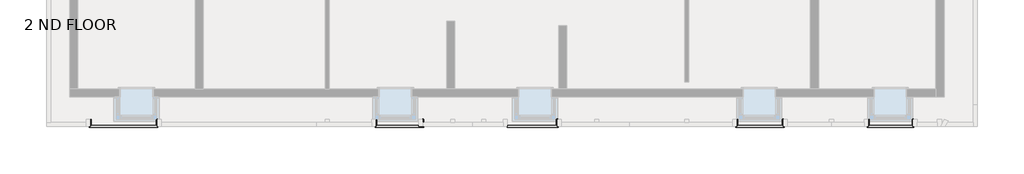
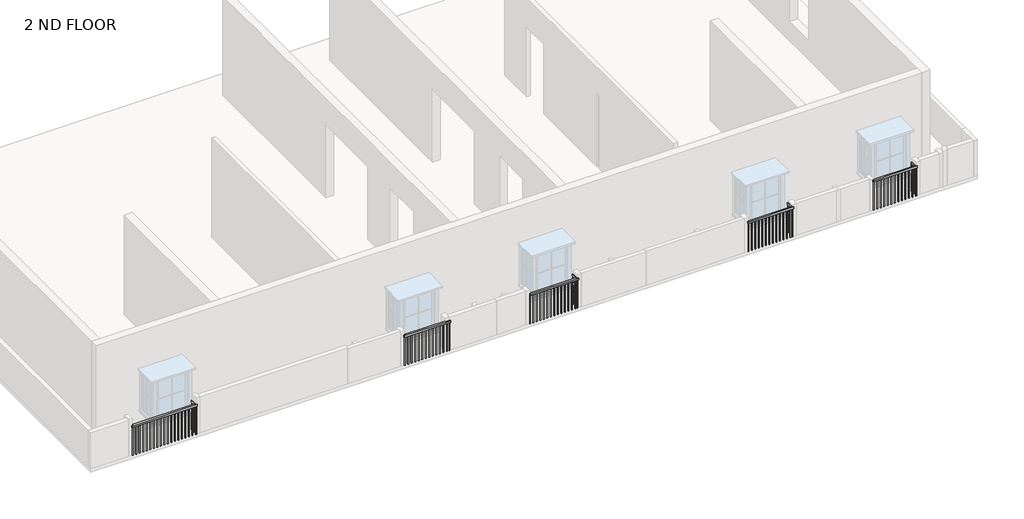
# One storey, part 3 of 7: 5 railings.
"""IFC4 building model written with IfcOpenShell, lengths in millimetres."""

from ifc_helpers import new_model, si_unit, frame, origin, place, context, project, spatial, polyline, outline, extrude, faceted_brep, element, save

model = new_model("IFC4")

# Units and contexts
model_context = context("Model", 3, world=origin())
ifc_project = project(units=[si_unit("LENGTHUNIT", "METRE", prefix="MILLI")], contexts=[model_context])

# Site, building, storey
site = spatial("IfcSite", under=ifc_project)
building = spatial("IfcBuilding", under=site)
storey = spatial("IfcBuildingStorey", under=building, Name="2 ND FLOOR", Elevation=6400.8)

# Railings
placement = place(None, origin())
element("IfcRailing", 1, ObjectType="Handrail - Rectangular", at=placement, inside=storey, context=model_context, shape_type="SolidModel", body=[
    faceted_brep([(-11856.9067989, -4623.6932193, 7315.2), (-11856.9067989, -4623.6932193, 7264.4), (-11907.7067989, -4623.6932193, 7264.4), (-11907.7067989, -4623.6932193, 7315.2), (-11856.9067989, -4801.4932661, 7315.2), (-11856.9067989, -4801.4932661, 7264.4), (-11907.7067989, -4852.2932661, 7264.4), (-11907.7067989, -4852.2932661, 7315.2), (-10071.3470335, -4801.4932661, 7315.2), (-10071.3470335, -4801.4932661, 7264.4), (-10020.5470335, -4852.2932661, 7264.4), (-10020.5470335, -4852.2932661, 7315.2), (-10071.3470335, -4623.6932193, 7315.2), (-10020.5470335, -4623.6932193, 7315.2), (-10020.5470335, -4623.6932193, 7264.4), (-10071.3470335, -4623.6932193, 7264.4)], [[[0, 1, 2, 3]], [[1, 0, 4, 5]], [[2, 1, 5, 6]], [[3, 2, 6, 7]], [[0, 3, 7, 4]], [[5, 4, 8, 9]], [[6, 5, 9, 10]], [[7, 6, 10, 11]], [[4, 7, 11, 8]], [[12, 13, 14, 15]], [[9, 8, 12, 15]], [[10, 9, 15, 14]], [[11, 10, 14, 13]], [[8, 11, 13, 12]]]),
    extrude(outline(polyline([(-10036.4220335, -4633.2182661), (-10055.4720335, -4633.2182661), (-10055.4720335, -4614.1682661), (-10036.4220335, -4614.1682661), (-10036.4220335, -4633.2182661)])), frame((0.0, 0.0, 6400.8), z_axis=(0.0, 0.0, 1.0), x_axis=(1.0, 0.0, 0.0)), (0.0, 0.0, 1.0), 863.6),
    extrude(outline(polyline([(-10036.4220335, -4734.8182661), (-10055.4720335, -4734.8182661), (-10055.4720335, -4715.7682661), (-10036.4220335, -4715.7682661), (-10036.4220335, -4734.8182661)])), frame((0.0, 0.0, 6400.8), z_axis=(0.0, 0.0, 1.0), x_axis=(1.0, 0.0, 0.0)), (0.0, 0.0, 1.0), 863.6),
    extrude(outline(polyline([(-10063.0317989, -4836.4182661), (-10063.0317989, -4817.3682661), (-10043.9817989, -4817.3682661), (-10043.9817989, -4836.4182661), (-10063.0317989, -4836.4182661)])), frame((0.0, 0.0, 6400.8), z_axis=(0.0, 0.0, 1.0), x_axis=(1.0, 0.0, 0.0)), (0.0, 0.0, 1.0), 863.6),
    extrude(outline(polyline([(-10164.6317989, -4836.4182661), (-10164.6317989, -4817.3682661), (-10145.5817989, -4817.3682661), (-10145.5817989, -4836.4182661), (-10164.6317989, -4836.4182661)])), frame((0.0, 0.0, 6400.8), z_axis=(0.0, 0.0, 1.0), x_axis=(1.0, 0.0, 0.0)), (0.0, 0.0, 1.0), 863.6),
    extrude(outline(polyline([(-10266.2317989, -4836.4182661), (-10266.2317989, -4817.3682661), (-10247.1817989, -4817.3682661), (-10247.1817989, -4836.4182661), (-10266.2317989, -4836.4182661)])), frame((0.0, 0.0, 6400.8), z_axis=(0.0, 0.0, 1.0), x_axis=(1.0, 0.0, 0.0)), (0.0, 0.0, 1.0), 863.6),
    extrude(outline(polyline([(-10367.8317989, -4836.4182661), (-10367.8317989, -4817.3682661), (-10348.7817989, -4817.3682661), (-10348.7817989, -4836.4182661), (-10367.8317989, -4836.4182661)])), frame((0.0, 0.0, 6400.8), z_axis=(0.0, 0.0, 1.0), x_axis=(1.0, 0.0, 0.0)), (0.0, 0.0, 1.0), 863.6),
    extrude(outline(polyline([(-10469.4317989, -4836.4182661), (-10469.4317989, -4817.3682661), (-10450.3817989, -4817.3682661), (-10450.3817989, -4836.4182661), (-10469.4317989, -4836.4182661)])), frame((0.0, 0.0, 6400.8), z_axis=(0.0, 0.0, 1.0), x_axis=(1.0, 0.0, 0.0)), (0.0, 0.0, 1.0), 863.6),
    extrude(outline(polyline([(-10571.0317989, -4836.4182661), (-10571.0317989, -4817.3682661), (-10551.9817989, -4817.3682661), (-10551.9817989, -4836.4182661), (-10571.0317989, -4836.4182661)])), frame((0.0, 0.0, 6400.8), z_axis=(0.0, 0.0, 1.0), x_axis=(1.0, 0.0, 0.0)), (0.0, 0.0, 1.0), 863.6),
    extrude(outline(polyline([(-10672.6317989, -4836.4182661), (-10672.6317989, -4817.3682661), (-10653.5817989, -4817.3682661), (-10653.5817989, -4836.4182661), (-10672.6317989, -4836.4182661)])), frame((0.0, 0.0, 6400.8), z_axis=(0.0, 0.0, 1.0), x_axis=(1.0, 0.0, 0.0)), (0.0, 0.0, 1.0), 863.6),
    extrude(outline(polyline([(-10774.2317989, -4836.4182661), (-10774.2317989, -4817.3682661), (-10755.1817989, -4817.3682661), (-10755.1817989, -4836.4182661), (-10774.2317989, -4836.4182661)])), frame((0.0, 0.0, 6400.8), z_axis=(0.0, 0.0, 1.0), x_axis=(1.0, 0.0, 0.0)), (0.0, 0.0, 1.0), 863.6),
    extrude(outline(polyline([(-10875.8317989, -4836.4182661), (-10875.8317989, -4817.3682661), (-10856.7817989, -4817.3682661), (-10856.7817989, -4836.4182661), (-10875.8317989, -4836.4182661)])), frame((0.0, 0.0, 6400.8), z_axis=(0.0, 0.0, 1.0), x_axis=(1.0, 0.0, 0.0)), (0.0, 0.0, 1.0), 863.6),
    extrude(outline(polyline([(-10977.4317989, -4836.4182661), (-10977.4317989, -4817.3682661), (-10958.3817989, -4817.3682661), (-10958.3817989, -4836.4182661), (-10977.4317989, -4836.4182661)])), frame((0.0, 0.0, 6400.8), z_axis=(0.0, 0.0, 1.0), x_axis=(1.0, 0.0, 0.0)), (0.0, 0.0, 1.0), 863.6),
    extrude(outline(polyline([(-11079.0317989, -4836.4182661), (-11079.0317989, -4817.3682661), (-11059.9817989, -4817.3682661), (-11059.9817989, -4836.4182661), (-11079.0317989, -4836.4182661)])), frame((0.0, 0.0, 6400.8), z_axis=(0.0, 0.0, 1.0), x_axis=(1.0, 0.0, 0.0)), (0.0, 0.0, 1.0), 863.6),
    extrude(outline(polyline([(-11180.6317989, -4836.4182661), (-11180.6317989, -4817.3682661), (-11161.5817989, -4817.3682661), (-11161.5817989, -4836.4182661), (-11180.6317989, -4836.4182661)])), frame((0.0, 0.0, 6400.8), z_axis=(0.0, 0.0, 1.0), x_axis=(1.0, 0.0, 0.0)), (0.0, 0.0, 1.0), 863.6),
    extrude(outline(polyline([(-11282.2317989, -4836.4182661), (-11282.2317989, -4817.3682661), (-11263.1817989, -4817.3682661), (-11263.1817989, -4836.4182661), (-11282.2317989, -4836.4182661)])), frame((0.0, 0.0, 6400.8), z_axis=(0.0, 0.0, 1.0), x_axis=(1.0, 0.0, 0.0)), (0.0, 0.0, 1.0), 863.6),
    extrude(outline(polyline([(-11383.8317989, -4836.4182661), (-11383.8317989, -4817.3682661), (-11364.7817989, -4817.3682661), (-11364.7817989, -4836.4182661), (-11383.8317989, -4836.4182661)])), frame((0.0, 0.0, 6400.8), z_axis=(0.0, 0.0, 1.0), x_axis=(1.0, 0.0, 0.0)), (0.0, 0.0, 1.0), 863.6),
    extrude(outline(polyline([(-11485.4317989, -4836.4182661), (-11485.4317989, -4817.3682661), (-11466.3817989, -4817.3682661), (-11466.3817989, -4836.4182661), (-11485.4317989, -4836.4182661)])), frame((0.0, 0.0, 6400.8), z_axis=(0.0, 0.0, 1.0), x_axis=(1.0, 0.0, 0.0)), (0.0, 0.0, 1.0), 863.6),
    extrude(outline(polyline([(-11587.0317989, -4836.4182661), (-11587.0317989, -4817.3682661), (-11567.9817989, -4817.3682661), (-11567.9817989, -4836.4182661), (-11587.0317989, -4836.4182661)])), frame((0.0, 0.0, 6400.8), z_axis=(0.0, 0.0, 1.0), x_axis=(1.0, 0.0, 0.0)), (0.0, 0.0, 1.0), 863.6),
    extrude(outline(polyline([(-11688.6317989, -4836.4182661), (-11688.6317989, -4817.3682661), (-11669.5817989, -4817.3682661), (-11669.5817989, -4836.4182661), (-11688.6317989, -4836.4182661)])), frame((0.0, 0.0, 6400.8), z_axis=(0.0, 0.0, 1.0), x_axis=(1.0, 0.0, 0.0)), (0.0, 0.0, 1.0), 863.6),
    extrude(outline(polyline([(-11790.2317989, -4836.4182661), (-11790.2317989, -4817.3682661), (-11771.1817989, -4817.3682661), (-11771.1817989, -4836.4182661), (-11790.2317989, -4836.4182661)])), frame((0.0, 0.0, 6400.8), z_axis=(0.0, 0.0, 1.0), x_axis=(1.0, 0.0, 0.0)), (0.0, 0.0, 1.0), 863.6),
    extrude(outline(polyline([(-11891.8317989, -4817.3682193), (-11872.7817989, -4817.3682193), (-11872.7817989, -4836.4182193), (-11891.8317989, -4836.4182193), (-11891.8317989, -4817.3682193)])), frame((0.0, 0.0, 6400.8), z_axis=(0.0, 0.0, 1.0), x_axis=(1.0, 0.0, 0.0)), (0.0, 0.0, 1.0), 863.6),
    extrude(outline(polyline([(-11891.8317989, -4715.7682193), (-11872.7817989, -4715.7682193), (-11872.7817989, -4734.8182193), (-11891.8317989, -4734.8182193), (-11891.8317989, -4715.7682193)])), frame((0.0, 0.0, 6400.8), z_axis=(0.0, 0.0, 1.0), x_axis=(1.0, 0.0, 0.0)), (0.0, 0.0, 1.0), 863.6),
    extrude(outline(polyline([(-10055.4720335, -4836.4182661), (-10055.4720335, -4817.3682661), (-10036.4220335, -4817.3682661), (-10036.4220335, -4836.4182661), (-10055.4720335, -4836.4182661)])), frame((0.0, 0.0, 6400.8), z_axis=(0.0, 0.0, 1.0), x_axis=(1.0, 0.0, 0.0)), (0.0, 0.0, 1.0), 863.6),
    extrude(outline(polyline([(-11891.8317989, -4817.3682661), (-11872.7817989, -4817.3682661), (-11872.7817989, -4836.4182661), (-11891.8317989, -4836.4182661), (-11891.8317989, -4817.3682661)])), frame((0.0, 0.0, 6400.8), z_axis=(0.0, 0.0, 1.0), x_axis=(1.0, 0.0, 0.0)), (0.0, 0.0, 1.0), 863.6),
    extrude(outline(polyline([(-10036.4220335, -4642.7432193), (-10055.4720335, -4642.7432193), (-10055.4720335, -4623.6932193), (-10036.4220335, -4623.6932193), (-10036.4220335, -4642.7432193)])), frame((0.0, 0.0, 6400.8), z_axis=(0.0, 0.0, 1.0), x_axis=(1.0, 0.0, 0.0)), (0.0, 0.0, 1.0), 863.6),
    extrude(outline(polyline([(-11891.8317989, -4623.6932193), (-11872.7817989, -4623.6932193), (-11872.7817989, -4642.7432193), (-11891.8317989, -4642.7432193), (-11891.8317989, -4623.6932193)])), frame((0.0, 0.0, 6400.8), z_axis=(0.0, 0.0, 1.0), x_axis=(1.0, 0.0, 0.0)), (0.0, 0.0, 1.0), 863.6),
])
element("IfcRailing", 2, ObjectType="Handrail - Rectangular", at=placement, inside=storey, context=model_context, shape_type="SolidModel", body=[
    faceted_brep([(-3995.0987995, -4623.6932193, 7315.2), (-3995.0987995, -4623.6932193, 7264.4), (-4045.8987995, -4623.6932193, 7264.4), (-4045.8987995, -4623.6932193, 7315.2), (-3995.0987995, -4801.4932661, 7315.2), (-3995.0987995, -4801.4932661, 7264.4), (-4045.8987995, -4852.2932661, 7264.4), (-4045.8987995, -4852.2932661, 7315.2), (-2750.4987995, -4801.4932661, 7315.2), (-2750.4987995, -4801.4932661, 7264.4), (-2699.6987995, -4852.2932661, 7264.4), (-2699.6987995, -4852.2932661, 7315.2), (-2750.4987995, -4623.6932193, 7315.2), (-2699.6987995, -4623.6932193, 7315.2), (-2699.6987995, -4623.6932193, 7264.4), (-2750.4987995, -4623.6932193, 7264.4)], [[[0, 1, 2, 3]], [[1, 0, 4, 5]], [[2, 1, 5, 6]], [[3, 2, 6, 7]], [[0, 3, 7, 4]], [[5, 4, 8, 9]], [[6, 5, 9, 10]], [[7, 6, 10, 11]], [[4, 7, 11, 8]], [[12, 13, 14, 15]], [[9, 8, 12, 15]], [[10, 9, 15, 14]], [[11, 10, 14, 13]], [[8, 11, 13, 12]]]),
    extrude(outline(polyline([(-2715.5737995, -4633.2182661), (-2734.6237995, -4633.2182661), (-2734.6237995, -4614.1682661), (-2715.5737995, -4614.1682661), (-2715.5737995, -4633.2182661)])), frame((0.0, 0.0, 6400.8), z_axis=(0.0, 0.0, 1.0), x_axis=(1.0, 0.0, 0.0)), (0.0, 0.0, 1.0), 863.6),
    extrude(outline(polyline([(-2715.5737995, -4734.8182661), (-2734.6237995, -4734.8182661), (-2734.6237995, -4715.7682661), (-2715.5737995, -4715.7682661), (-2715.5737995, -4734.8182661)])), frame((0.0, 0.0, 6400.8), z_axis=(0.0, 0.0, 1.0), x_axis=(1.0, 0.0, 0.0)), (0.0, 0.0, 1.0), 863.6),
    extrude(outline(polyline([(-2810.8237995, -4836.4182661), (-2810.8237995, -4817.3682661), (-2791.7737995, -4817.3682661), (-2791.7737995, -4836.4182661), (-2810.8237995, -4836.4182661)])), frame((0.0, 0.0, 6400.8), z_axis=(0.0, 0.0, 1.0), x_axis=(1.0, 0.0, 0.0)), (0.0, 0.0, 1.0), 863.6),
    extrude(outline(polyline([(-2912.4237995, -4836.4182661), (-2912.4237995, -4817.3682661), (-2893.3737995, -4817.3682661), (-2893.3737995, -4836.4182661), (-2912.4237995, -4836.4182661)])), frame((0.0, 0.0, 6400.8), z_axis=(0.0, 0.0, 1.0), x_axis=(1.0, 0.0, 0.0)), (0.0, 0.0, 1.0), 863.6),
    extrude(outline(polyline([(-3014.0237995, -4836.4182661), (-3014.0237995, -4817.3682661), (-2994.9737995, -4817.3682661), (-2994.9737995, -4836.4182661), (-3014.0237995, -4836.4182661)])), frame((0.0, 0.0, 6400.8), z_axis=(0.0, 0.0, 1.0), x_axis=(1.0, 0.0, 0.0)), (0.0, 0.0, 1.0), 863.6),
    extrude(outline(polyline([(-3115.6237995, -4836.4182661), (-3115.6237995, -4817.3682661), (-3096.5737995, -4817.3682661), (-3096.5737995, -4836.4182661), (-3115.6237995, -4836.4182661)])), frame((0.0, 0.0, 6400.8), z_axis=(0.0, 0.0, 1.0), x_axis=(1.0, 0.0, 0.0)), (0.0, 0.0, 1.0), 863.6),
    extrude(outline(polyline([(-3217.2237995, -4836.4182661), (-3217.2237995, -4817.3682661), (-3198.1737995, -4817.3682661), (-3198.1737995, -4836.4182661), (-3217.2237995, -4836.4182661)])), frame((0.0, 0.0, 6400.8), z_axis=(0.0, 0.0, 1.0), x_axis=(1.0, 0.0, 0.0)), (0.0, 0.0, 1.0), 863.6),
    extrude(outline(polyline([(-3318.8237995, -4836.4182661), (-3318.8237995, -4817.3682661), (-3299.7737995, -4817.3682661), (-3299.7737995, -4836.4182661), (-3318.8237995, -4836.4182661)])), frame((0.0, 0.0, 6400.8), z_axis=(0.0, 0.0, 1.0), x_axis=(1.0, 0.0, 0.0)), (0.0, 0.0, 1.0), 863.6),
    extrude(outline(polyline([(-3420.4237995, -4836.4182661), (-3420.4237995, -4817.3682661), (-3401.3737995, -4817.3682661), (-3401.3737995, -4836.4182661), (-3420.4237995, -4836.4182661)])), frame((0.0, 0.0, 6400.8), z_axis=(0.0, 0.0, 1.0), x_axis=(1.0, 0.0, 0.0)), (0.0, 0.0, 1.0), 863.6),
    extrude(outline(polyline([(-3522.0237995, -4836.4182661), (-3522.0237995, -4817.3682661), (-3502.9737995, -4817.3682661), (-3502.9737995, -4836.4182661), (-3522.0237995, -4836.4182661)])), frame((0.0, 0.0, 6400.8), z_axis=(0.0, 0.0, 1.0), x_axis=(1.0, 0.0, 0.0)), (0.0, 0.0, 1.0), 863.6),
    extrude(outline(polyline([(-3623.6237995, -4836.4182661), (-3623.6237995, -4817.3682661), (-3604.5737995, -4817.3682661), (-3604.5737995, -4836.4182661), (-3623.6237995, -4836.4182661)])), frame((0.0, 0.0, 6400.8), z_axis=(0.0, 0.0, 1.0), x_axis=(1.0, 0.0, 0.0)), (0.0, 0.0, 1.0), 863.6),
    extrude(outline(polyline([(-3725.2237995, -4836.4182661), (-3725.2237995, -4817.3682661), (-3706.1737995, -4817.3682661), (-3706.1737995, -4836.4182661), (-3725.2237995, -4836.4182661)])), frame((0.0, 0.0, 6400.8), z_axis=(0.0, 0.0, 1.0), x_axis=(1.0, 0.0, 0.0)), (0.0, 0.0, 1.0), 863.6),
    extrude(outline(polyline([(-3826.8237995, -4836.4182661), (-3826.8237995, -4817.3682661), (-3807.7737995, -4817.3682661), (-3807.7737995, -4836.4182661), (-3826.8237995, -4836.4182661)])), frame((0.0, 0.0, 6400.8), z_axis=(0.0, 0.0, 1.0), x_axis=(1.0, 0.0, 0.0)), (0.0, 0.0, 1.0), 863.6),
    extrude(outline(polyline([(-3928.4237995, -4836.4182661), (-3928.4237995, -4817.3682661), (-3909.3737995, -4817.3682661), (-3909.3737995, -4836.4182661), (-3928.4237995, -4836.4182661)])), frame((0.0, 0.0, 6400.8), z_axis=(0.0, 0.0, 1.0), x_axis=(1.0, 0.0, 0.0)), (0.0, 0.0, 1.0), 863.6),
    extrude(outline(polyline([(-4030.0237995, -4817.3682193), (-4010.9737995, -4817.3682193), (-4010.9737995, -4836.4182193), (-4030.0237995, -4836.4182193), (-4030.0237995, -4817.3682193)])), frame((0.0, 0.0, 6400.8), z_axis=(0.0, 0.0, 1.0), x_axis=(1.0, 0.0, 0.0)), (0.0, 0.0, 1.0), 863.6),
    extrude(outline(polyline([(-4030.0237995, -4715.7682193), (-4010.9737995, -4715.7682193), (-4010.9737995, -4734.8182193), (-4030.0237995, -4734.8182193), (-4030.0237995, -4715.7682193)])), frame((0.0, 0.0, 6400.8), z_axis=(0.0, 0.0, 1.0), x_axis=(1.0, 0.0, 0.0)), (0.0, 0.0, 1.0), 863.6),
    extrude(outline(polyline([(-2734.6237995, -4836.4182661), (-2734.6237995, -4817.3682661), (-2715.5737995, -4817.3682661), (-2715.5737995, -4836.4182661), (-2734.6237995, -4836.4182661)])), frame((0.0, 0.0, 6400.8), z_axis=(0.0, 0.0, 1.0), x_axis=(1.0, 0.0, 0.0)), (0.0, 0.0, 1.0), 863.6),
    extrude(outline(polyline([(-4030.0237995, -4817.3682661), (-4010.9737995, -4817.3682661), (-4010.9737995, -4836.4182661), (-4030.0237995, -4836.4182661), (-4030.0237995, -4817.3682661)])), frame((0.0, 0.0, 6400.8), z_axis=(0.0, 0.0, 1.0), x_axis=(1.0, 0.0, 0.0)), (0.0, 0.0, 1.0), 863.6),
    extrude(outline(polyline([(-2715.5737995, -4642.7432193), (-2734.6237995, -4642.7432193), (-2734.6237995, -4623.6932193), (-2715.5737995, -4623.6932193), (-2715.5737995, -4642.7432193)])), frame((0.0, 0.0, 6400.8), z_axis=(0.0, 0.0, 1.0), x_axis=(1.0, 0.0, 0.0)), (0.0, 0.0, 1.0), 863.6),
    extrude(outline(polyline([(-4030.0237995, -4623.6932193), (-4010.9737995, -4623.6932193), (-4010.9737995, -4642.7432193), (-4030.0237995, -4642.7432193), (-4030.0237995, -4623.6932193)])), frame((0.0, 0.0, 6400.8), z_axis=(0.0, 0.0, 1.0), x_axis=(1.0, 0.0, 0.0)), (0.0, 0.0, 1.0), 863.6),
])
element("IfcRailing", 3, ObjectType="Handrail - Rectangular", at=placement, inside=storey, context=model_context, shape_type="SolidModel", body=[
    faceted_brep([(-406.2065315, -4801.4932661, 7315.2), (-406.2065315, -4801.4932661, 7264.4), (-406.2065315, -4852.2932661, 7264.4), (-406.2065315, -4852.2932661, 7315.2), (944.6932011, -4801.4932661, 7315.2), (944.6932011, -4801.4932661, 7264.4), (995.4932011, -4852.2932661, 7264.4), (995.4932011, -4852.2932661, 7315.2), (944.6932011, -4623.6932193, 7315.2), (995.4932011, -4623.6932193, 7315.2), (995.4932011, -4623.6932193, 7264.4), (944.6932011, -4623.6932193, 7264.4)], [[[0, 1, 2, 3]], [[1, 0, 4, 5]], [[2, 1, 5, 6]], [[3, 2, 6, 7]], [[0, 3, 7, 4]], [[8, 9, 10, 11]], [[5, 4, 8, 11]], [[6, 5, 11, 10]], [[7, 6, 10, 9]], [[4, 7, 9, 8]]]),
    extrude(outline(polyline([(979.6182011, -4633.2182661), (960.5682011, -4633.2182661), (960.5682011, -4614.1682661), (979.6182011, -4614.1682661), (979.6182011, -4633.2182661)])), frame((0.0, 0.0, 6400.8), z_axis=(0.0, 0.0, 1.0), x_axis=(1.0, 0.0, 0.0)), (0.0, 0.0, 1.0), 863.6),
    extrude(outline(polyline([(979.6182011, -4734.8182661), (960.5682011, -4734.8182661), (960.5682011, -4715.7682661), (979.6182011, -4715.7682661), (979.6182011, -4734.8182661)])), frame((0.0, 0.0, 6400.8), z_axis=(0.0, 0.0, 1.0), x_axis=(1.0, 0.0, 0.0)), (0.0, 0.0, 1.0), 863.6),
    extrude(outline(polyline([(905.0684685, -4836.4182661), (905.0684685, -4817.3682661), (924.1184685, -4817.3682661), (924.1184685, -4836.4182661), (905.0684685, -4836.4182661)])), frame((0.0, 0.0, 6400.8), z_axis=(0.0, 0.0, 1.0), x_axis=(1.0, 0.0, 0.0)), (0.0, 0.0, 1.0), 863.6),
    extrude(outline(polyline([(803.4684685, -4836.4182661), (803.4684685, -4817.3682661), (822.5184685, -4817.3682661), (822.5184685, -4836.4182661), (803.4684685, -4836.4182661)])), frame((0.0, 0.0, 6400.8), z_axis=(0.0, 0.0, 1.0), x_axis=(1.0, 0.0, 0.0)), (0.0, 0.0, 1.0), 863.6),
    extrude(outline(polyline([(701.8684685, -4836.4182661), (701.8684685, -4817.3682661), (720.9184685, -4817.3682661), (720.9184685, -4836.4182661), (701.8684685, -4836.4182661)])), frame((0.0, 0.0, 6400.8), z_axis=(0.0, 0.0, 1.0), x_axis=(1.0, 0.0, 0.0)), (0.0, 0.0, 1.0), 863.6),
    extrude(outline(polyline([(600.2684685, -4836.4182661), (600.2684685, -4817.3682661), (619.3184685, -4817.3682661), (619.3184685, -4836.4182661), (600.2684685, -4836.4182661)])), frame((0.0, 0.0, 6400.8), z_axis=(0.0, 0.0, 1.0), x_axis=(1.0, 0.0, 0.0)), (0.0, 0.0, 1.0), 863.6),
    extrude(outline(polyline([(498.6684685, -4836.4182661), (498.6684685, -4817.3682661), (517.7184685, -4817.3682661), (517.7184685, -4836.4182661), (498.6684685, -4836.4182661)])), frame((0.0, 0.0, 6400.8), z_axis=(0.0, 0.0, 1.0), x_axis=(1.0, 0.0, 0.0)), (0.0, 0.0, 1.0), 863.6),
    extrude(outline(polyline([(397.0684685, -4836.4182661), (397.0684685, -4817.3682661), (416.1184685, -4817.3682661), (416.1184685, -4836.4182661), (397.0684685, -4836.4182661)])), frame((0.0, 0.0, 6400.8), z_axis=(0.0, 0.0, 1.0), x_axis=(1.0, 0.0, 0.0)), (0.0, 0.0, 1.0), 863.6),
    extrude(outline(polyline([(295.4684685, -4836.4182661), (295.4684685, -4817.3682661), (314.5184685, -4817.3682661), (314.5184685, -4836.4182661), (295.4684685, -4836.4182661)])), frame((0.0, 0.0, 6400.8), z_axis=(0.0, 0.0, 1.0), x_axis=(1.0, 0.0, 0.0)), (0.0, 0.0, 1.0), 863.6),
    extrude(outline(polyline([(193.8684685, -4836.4182661), (193.8684685, -4817.3682661), (212.9184685, -4817.3682661), (212.9184685, -4836.4182661), (193.8684685, -4836.4182661)])), frame((0.0, 0.0, 6400.8), z_axis=(0.0, 0.0, 1.0), x_axis=(1.0, 0.0, 0.0)), (0.0, 0.0, 1.0), 863.6),
    extrude(outline(polyline([(92.2684685, -4836.4182661), (92.2684685, -4817.3682661), (111.3184685, -4817.3682661), (111.3184685, -4836.4182661), (92.2684685, -4836.4182661)])), frame((0.0, 0.0, 6400.8), z_axis=(0.0, 0.0, 1.0), x_axis=(1.0, 0.0, 0.0)), (0.0, 0.0, 1.0), 863.6),
    extrude(outline(polyline([(-9.3315315, -4836.4182661), (-9.3315315, -4817.3682661), (9.7184685, -4817.3682661), (9.7184685, -4836.4182661), (-9.3315315, -4836.4182661)])), frame((0.0, 0.0, 6400.8), z_axis=(0.0, 0.0, 1.0), x_axis=(1.0, 0.0, 0.0)), (0.0, 0.0, 1.0), 863.6),
    extrude(outline(polyline([(-110.9315315, -4836.4182661), (-110.9315315, -4817.3682661), (-91.8815315, -4817.3682661), (-91.8815315, -4836.4182661), (-110.9315315, -4836.4182661)])), frame((0.0, 0.0, 6400.8), z_axis=(0.0, 0.0, 1.0), x_axis=(1.0, 0.0, 0.0)), (0.0, 0.0, 1.0), 863.6),
    extrude(outline(polyline([(-212.5315315, -4836.4182661), (-212.5315315, -4817.3682661), (-193.4815315, -4817.3682661), (-193.4815315, -4836.4182661), (-212.5315315, -4836.4182661)])), frame((0.0, 0.0, 6400.8), z_axis=(0.0, 0.0, 1.0), x_axis=(1.0, 0.0, 0.0)), (0.0, 0.0, 1.0), 863.6),
    extrude(outline(polyline([(-314.1315315, -4836.4182661), (-314.1315315, -4817.3682661), (-295.0815315, -4817.3682661), (-295.0815315, -4836.4182661), (-314.1315315, -4836.4182661)])), frame((0.0, 0.0, 6400.8), z_axis=(0.0, 0.0, 1.0), x_axis=(1.0, 0.0, 0.0)), (0.0, 0.0, 1.0), 863.6),
    extrude(outline(polyline([(960.5682011, -4836.4182661), (960.5682011, -4817.3682661), (979.6182011, -4817.3682661), (979.6182011, -4836.4182661), (960.5682011, -4836.4182661)])), frame((0.0, 0.0, 6400.8), z_axis=(0.0, 0.0, 1.0), x_axis=(1.0, 0.0, 0.0)), (0.0, 0.0, 1.0), 863.6),
    extrude(outline(polyline([(979.6182011, -4642.7432193), (960.5682011, -4642.7432193), (960.5682011, -4623.6932193), (979.6182011, -4623.6932193), (979.6182011, -4642.7432193)])), frame((0.0, 0.0, 6400.8), z_axis=(0.0, 0.0, 1.0), x_axis=(1.0, 0.0, 0.0)), (0.0, 0.0, 1.0), 863.6),
    extrude(outline(polyline([(-406.2065315, -4836.4182661), (-406.2065315, -4817.3682661), (-387.1565315, -4817.3682661), (-387.1565315, -4836.4182661), (-406.2065315, -4836.4182661)])), frame((0.0, 0.0, 6400.8), z_axis=(0.0, 0.0, 1.0), x_axis=(1.0, 0.0, 0.0)), (0.0, 0.0, 1.0), 863.6),
])
element("IfcRailing", 4, ObjectType="Handrail - Rectangular", at=placement, inside=storey, context=model_context, shape_type="SolidModel", body=[
    faceted_brep([(5942.6512082, -4623.6932193, 7315.2), (5942.6512082, -4623.6932193, 7264.4), (5891.8512082, -4623.6932193, 7264.4), (5891.8512082, -4623.6932193, 7315.2), (5942.6512082, -4801.4932661, 7315.2), (5942.6512082, -4801.4932661, 7264.4), (5891.8512082, -4852.2932661, 7264.4), (5891.8512082, -4852.2932661, 7315.2), (7164.9011643, -4801.4932661, 7315.2), (7164.9011643, -4801.4932661, 7264.4), (7215.7011643, -4852.2932661, 7264.4), (7215.7011643, -4852.2932661, 7315.2), (7164.9011643, -4623.6932193, 7315.2), (7215.7011643, -4623.6932193, 7315.2), (7215.7011643, -4623.6932193, 7264.4), (7164.9011643, -4623.6932193, 7264.4)], [[[0, 1, 2, 3]], [[1, 0, 4, 5]], [[2, 1, 5, 6]], [[3, 2, 6, 7]], [[0, 3, 7, 4]], [[5, 4, 8, 9]], [[6, 5, 9, 10]], [[7, 6, 10, 11]], [[4, 7, 11, 8]], [[12, 13, 14, 15]], [[9, 8, 12, 15]], [[10, 9, 15, 14]], [[11, 10, 14, 13]], [[8, 11, 13, 12]]]),
    extrude(outline(polyline([(7199.8261643, -4633.2182661), (7180.7761643, -4633.2182661), (7180.7761643, -4614.1682661), (7199.8261643, -4614.1682661), (7199.8261643, -4633.2182661)])), frame((0.0, 0.0, 6400.8), z_axis=(0.0, 0.0, 1.0), x_axis=(1.0, 0.0, 0.0)), (0.0, 0.0, 1.0), 863.6),
    extrude(outline(polyline([(7199.8261643, -4734.8182661), (7180.7761643, -4734.8182661), (7180.7761643, -4715.7682661), (7199.8261643, -4715.7682661), (7199.8261643, -4734.8182661)])), frame((0.0, 0.0, 6400.8), z_axis=(0.0, 0.0, 1.0), x_axis=(1.0, 0.0, 0.0)), (0.0, 0.0, 1.0), 863.6),
    extrude(outline(polyline([(7126.9262082, -4836.4182661), (7126.9262082, -4817.3682661), (7145.9762082, -4817.3682661), (7145.9762082, -4836.4182661), (7126.9262082, -4836.4182661)])), frame((0.0, 0.0, 6400.8), z_axis=(0.0, 0.0, 1.0), x_axis=(1.0, 0.0, 0.0)), (0.0, 0.0, 1.0), 863.6),
    extrude(outline(polyline([(7025.3262082, -4836.4182661), (7025.3262082, -4817.3682661), (7044.3762082, -4817.3682661), (7044.3762082, -4836.4182661), (7025.3262082, -4836.4182661)])), frame((0.0, 0.0, 6400.8), z_axis=(0.0, 0.0, 1.0), x_axis=(1.0, 0.0, 0.0)), (0.0, 0.0, 1.0), 863.6),
    extrude(outline(polyline([(6923.7262082, -4836.4182661), (6923.7262082, -4817.3682661), (6942.7762082, -4817.3682661), (6942.7762082, -4836.4182661), (6923.7262082, -4836.4182661)])), frame((0.0, 0.0, 6400.8), z_axis=(0.0, 0.0, 1.0), x_axis=(1.0, 0.0, 0.0)), (0.0, 0.0, 1.0), 863.6),
    extrude(outline(polyline([(6822.1262082, -4836.4182661), (6822.1262082, -4817.3682661), (6841.1762082, -4817.3682661), (6841.1762082, -4836.4182661), (6822.1262082, -4836.4182661)])), frame((0.0, 0.0, 6400.8), z_axis=(0.0, 0.0, 1.0), x_axis=(1.0, 0.0, 0.0)), (0.0, 0.0, 1.0), 863.6),
    extrude(outline(polyline([(6720.5262082, -4836.4182661), (6720.5262082, -4817.3682661), (6739.5762082, -4817.3682661), (6739.5762082, -4836.4182661), (6720.5262082, -4836.4182661)])), frame((0.0, 0.0, 6400.8), z_axis=(0.0, 0.0, 1.0), x_axis=(1.0, 0.0, 0.0)), (0.0, 0.0, 1.0), 863.6),
    extrude(outline(polyline([(6618.9262082, -4836.4182661), (6618.9262082, -4817.3682661), (6637.9762082, -4817.3682661), (6637.9762082, -4836.4182661), (6618.9262082, -4836.4182661)])), frame((0.0, 0.0, 6400.8), z_axis=(0.0, 0.0, 1.0), x_axis=(1.0, 0.0, 0.0)), (0.0, 0.0, 1.0), 863.6),
    extrude(outline(polyline([(6517.3262082, -4836.4182661), (6517.3262082, -4817.3682661), (6536.3762082, -4817.3682661), (6536.3762082, -4836.4182661), (6517.3262082, -4836.4182661)])), frame((0.0, 0.0, 6400.8), z_axis=(0.0, 0.0, 1.0), x_axis=(1.0, 0.0, 0.0)), (0.0, 0.0, 1.0), 863.6),
    extrude(outline(polyline([(6415.7262082, -4836.4182661), (6415.7262082, -4817.3682661), (6434.7762082, -4817.3682661), (6434.7762082, -4836.4182661), (6415.7262082, -4836.4182661)])), frame((0.0, 0.0, 6400.8), z_axis=(0.0, 0.0, 1.0), x_axis=(1.0, 0.0, 0.0)), (0.0, 0.0, 1.0), 863.6),
    extrude(outline(polyline([(6314.1262082, -4836.4182661), (6314.1262082, -4817.3682661), (6333.1762082, -4817.3682661), (6333.1762082, -4836.4182661), (6314.1262082, -4836.4182661)])), frame((0.0, 0.0, 6400.8), z_axis=(0.0, 0.0, 1.0), x_axis=(1.0, 0.0, 0.0)), (0.0, 0.0, 1.0), 863.6),
    extrude(outline(polyline([(6212.5262082, -4836.4182661), (6212.5262082, -4817.3682661), (6231.5762082, -4817.3682661), (6231.5762082, -4836.4182661), (6212.5262082, -4836.4182661)])), frame((0.0, 0.0, 6400.8), z_axis=(0.0, 0.0, 1.0), x_axis=(1.0, 0.0, 0.0)), (0.0, 0.0, 1.0), 863.6),
    extrude(outline(polyline([(6110.9262082, -4836.4182661), (6110.9262082, -4817.3682661), (6129.9762082, -4817.3682661), (6129.9762082, -4836.4182661), (6110.9262082, -4836.4182661)])), frame((0.0, 0.0, 6400.8), z_axis=(0.0, 0.0, 1.0), x_axis=(1.0, 0.0, 0.0)), (0.0, 0.0, 1.0), 863.6),
    extrude(outline(polyline([(6009.3262082, -4836.4182661), (6009.3262082, -4817.3682661), (6028.3762082, -4817.3682661), (6028.3762082, -4836.4182661), (6009.3262082, -4836.4182661)])), frame((0.0, 0.0, 6400.8), z_axis=(0.0, 0.0, 1.0), x_axis=(1.0, 0.0, 0.0)), (0.0, 0.0, 1.0), 863.6),
    extrude(outline(polyline([(5907.7262082, -4817.3682193), (5926.7762082, -4817.3682193), (5926.7762082, -4836.4182193), (5907.7262082, -4836.4182193), (5907.7262082, -4817.3682193)])), frame((0.0, 0.0, 6400.8), z_axis=(0.0, 0.0, 1.0), x_axis=(1.0, 0.0, 0.0)), (0.0, 0.0, 1.0), 863.6),
    extrude(outline(polyline([(5907.7262082, -4715.7682193), (5926.7762082, -4715.7682193), (5926.7762082, -4734.8182193), (5907.7262082, -4734.8182193), (5907.7262082, -4715.7682193)])), frame((0.0, 0.0, 6400.8), z_axis=(0.0, 0.0, 1.0), x_axis=(1.0, 0.0, 0.0)), (0.0, 0.0, 1.0), 863.6),
    extrude(outline(polyline([(7180.7761643, -4836.4182661), (7180.7761643, -4817.3682661), (7199.8261643, -4817.3682661), (7199.8261643, -4836.4182661), (7180.7761643, -4836.4182661)])), frame((0.0, 0.0, 6400.8), z_axis=(0.0, 0.0, 1.0), x_axis=(1.0, 0.0, 0.0)), (0.0, 0.0, 1.0), 863.6),
    extrude(outline(polyline([(5907.7262082, -4817.3682661), (5926.7762082, -4817.3682661), (5926.7762082, -4836.4182661), (5907.7262082, -4836.4182661), (5907.7262082, -4817.3682661)])), frame((0.0, 0.0, 6400.8), z_axis=(0.0, 0.0, 1.0), x_axis=(1.0, 0.0, 0.0)), (0.0, 0.0, 1.0), 863.6),
    extrude(outline(polyline([(7199.8261643, -4642.7432193), (7180.7761643, -4642.7432193), (7180.7761643, -4623.6932193), (7199.8261643, -4623.6932193), (7199.8261643, -4642.7432193)])), frame((0.0, 0.0, 6400.8), z_axis=(0.0, 0.0, 1.0), x_axis=(1.0, 0.0, 0.0)), (0.0, 0.0, 1.0), 863.6),
    extrude(outline(polyline([(5907.7262082, -4623.6932193), (5926.7762082, -4623.6932193), (5926.7762082, -4642.7432193), (5907.7262082, -4642.7432193), (5907.7262082, -4623.6932193)])), frame((0.0, 0.0, 6400.8), z_axis=(0.0, 0.0, 1.0), x_axis=(1.0, 0.0, 0.0)), (0.0, 0.0, 1.0), 863.6),
])
element("IfcRailing", 5, ObjectType="Handrail - Rectangular", at=placement, inside=storey, context=model_context, shape_type="SolidModel", body=[
    faceted_brep([(9562.1512082, -4623.6932193, 7315.2), (9562.1512082, -4623.6932193, 7264.4), (9511.3512082, -4623.6932193, 7264.4), (9511.3512082, -4623.6932193, 7315.2), (9562.1512082, -4801.4932661, 7315.2), (9562.1512082, -4801.4932661, 7264.4), (9511.3512082, -4852.2932661, 7264.4), (9511.3512082, -4852.2932661, 7315.2), (10738.7617205, -4801.4932661, 7315.2), (10738.7617205, -4801.4932661, 7264.4), (10789.5617205, -4852.2932661, 7264.4), (10789.5617205, -4852.2932661, 7315.2), (10738.7617205, -4623.6932193, 7315.2), (10789.5617205, -4623.6932193, 7315.2), (10789.5617205, -4623.6932193, 7264.4), (10738.7617205, -4623.6932193, 7264.4)], [[[0, 1, 2, 3]], [[1, 0, 4, 5]], [[2, 1, 5, 6]], [[3, 2, 6, 7]], [[0, 3, 7, 4]], [[5, 4, 8, 9]], [[6, 5, 9, 10]], [[7, 6, 10, 11]], [[4, 7, 11, 8]], [[12, 13, 14, 15]], [[9, 8, 12, 15]], [[10, 9, 15, 14]], [[11, 10, 14, 13]], [[8, 11, 13, 12]]]),
    extrude(outline(polyline([(10754.6367205, -4633.2182661), (10754.6367205, -4614.1682661), (10773.6867205, -4614.1682661), (10773.6867205, -4633.2182661), (10754.6367205, -4633.2182661)])), frame((0.0, 0.0, 6400.8), z_axis=(0.0, 0.0, 1.0), x_axis=(1.0, 0.0, 0.0)), (0.0, 0.0, 1.0), 863.6),
    extrude(outline(polyline([(10754.6367205, -4734.8182661), (10754.6367205, -4715.7682661), (10773.6867205, -4715.7682661), (10773.6867205, -4734.8182661), (10754.6367205, -4734.8182661)])), frame((0.0, 0.0, 6400.8), z_axis=(0.0, 0.0, 1.0), x_axis=(1.0, 0.0, 0.0)), (0.0, 0.0, 1.0), 863.6),
    extrude(outline(polyline([(10746.4262082, -4817.3682661), (10765.4762082, -4817.3682661), (10765.4762082, -4836.4182661), (10746.4262082, -4836.4182661), (10746.4262082, -4817.3682661)])), frame((0.0, 0.0, 6400.8), z_axis=(0.0, 0.0, 1.0), x_axis=(1.0, 0.0, 0.0)), (0.0, 0.0, 1.0), 863.6),
    extrude(outline(polyline([(10644.8262082, -4817.3682661), (10663.8762082, -4817.3682661), (10663.8762082, -4836.4182661), (10644.8262082, -4836.4182661), (10644.8262082, -4817.3682661)])), frame((0.0, 0.0, 6400.8), z_axis=(0.0, 0.0, 1.0), x_axis=(1.0, 0.0, 0.0)), (0.0, 0.0, 1.0), 863.6),
    extrude(outline(polyline([(10543.2262082, -4817.3682661), (10562.2762082, -4817.3682661), (10562.2762082, -4836.4182661), (10543.2262082, -4836.4182661), (10543.2262082, -4817.3682661)])), frame((0.0, 0.0, 6400.8), z_axis=(0.0, 0.0, 1.0), x_axis=(1.0, 0.0, 0.0)), (0.0, 0.0, 1.0), 863.6),
    extrude(outline(polyline([(10441.6262082, -4817.3682661), (10460.6762082, -4817.3682661), (10460.6762082, -4836.4182661), (10441.6262082, -4836.4182661), (10441.6262082, -4817.3682661)])), frame((0.0, 0.0, 6400.8), z_axis=(0.0, 0.0, 1.0), x_axis=(1.0, 0.0, 0.0)), (0.0, 0.0, 1.0), 863.6),
    extrude(outline(polyline([(10340.0262082, -4817.3682661), (10359.0762082, -4817.3682661), (10359.0762082, -4836.4182661), (10340.0262082, -4836.4182661), (10340.0262082, -4817.3682661)])), frame((0.0, 0.0, 6400.8), z_axis=(0.0, 0.0, 1.0), x_axis=(1.0, 0.0, 0.0)), (0.0, 0.0, 1.0), 863.6),
    extrude(outline(polyline([(10238.4262082, -4817.3682661), (10257.4762082, -4817.3682661), (10257.4762082, -4836.4182661), (10238.4262082, -4836.4182661), (10238.4262082, -4817.3682661)])), frame((0.0, 0.0, 6400.8), z_axis=(0.0, 0.0, 1.0), x_axis=(1.0, 0.0, 0.0)), (0.0, 0.0, 1.0), 863.6),
    extrude(outline(polyline([(10136.8262082, -4817.3682661), (10155.8762082, -4817.3682661), (10155.8762082, -4836.4182661), (10136.8262082, -4836.4182661), (10136.8262082, -4817.3682661)])), frame((0.0, 0.0, 6400.8), z_axis=(0.0, 0.0, 1.0), x_axis=(1.0, 0.0, 0.0)), (0.0, 0.0, 1.0), 863.6),
    extrude(outline(polyline([(10035.2262082, -4817.3682661), (10054.2762082, -4817.3682661), (10054.2762082, -4836.4182661), (10035.2262082, -4836.4182661), (10035.2262082, -4817.3682661)])), frame((0.0, 0.0, 6400.8), z_axis=(0.0, 0.0, 1.0), x_axis=(1.0, 0.0, 0.0)), (0.0, 0.0, 1.0), 863.6),
    extrude(outline(polyline([(9933.6262082, -4817.3682661), (9952.6762082, -4817.3682661), (9952.6762082, -4836.4182661), (9933.6262082, -4836.4182661), (9933.6262082, -4817.3682661)])), frame((0.0, 0.0, 6400.8), z_axis=(0.0, 0.0, 1.0), x_axis=(1.0, 0.0, 0.0)), (0.0, 0.0, 1.0), 863.6),
    extrude(outline(polyline([(9832.0262082, -4817.3682661), (9851.0762082, -4817.3682661), (9851.0762082, -4836.4182661), (9832.0262082, -4836.4182661), (9832.0262082, -4817.3682661)])), frame((0.0, 0.0, 6400.8), z_axis=(0.0, 0.0, 1.0), x_axis=(1.0, 0.0, 0.0)), (0.0, 0.0, 1.0), 863.6),
    extrude(outline(polyline([(9730.4262082, -4817.3682661), (9749.4762082, -4817.3682661), (9749.4762082, -4836.4182661), (9730.4262082, -4836.4182661), (9730.4262082, -4817.3682661)])), frame((0.0, 0.0, 6400.8), z_axis=(0.0, 0.0, 1.0), x_axis=(1.0, 0.0, 0.0)), (0.0, 0.0, 1.0), 863.6),
    extrude(outline(polyline([(9628.8262082, -4817.3682661), (9647.8762082, -4817.3682661), (9647.8762082, -4836.4182661), (9628.8262082, -4836.4182661), (9628.8262082, -4817.3682661)])), frame((0.0, 0.0, 6400.8), z_axis=(0.0, 0.0, 1.0), x_axis=(1.0, 0.0, 0.0)), (0.0, 0.0, 1.0), 863.6),
    extrude(outline(polyline([(9546.2762082, -4817.3682193), (9546.2762082, -4836.4182193), (9527.2262082, -4836.4182193), (9527.2262082, -4817.3682193), (9546.2762082, -4817.3682193)])), frame((0.0, 0.0, 6400.8), z_axis=(0.0, 0.0, 1.0), x_axis=(1.0, 0.0, 0.0)), (0.0, 0.0, 1.0), 863.6),
    extrude(outline(polyline([(9546.2762082, -4715.7682193), (9546.2762082, -4734.8182193), (9527.2262082, -4734.8182193), (9527.2262082, -4715.7682193), (9546.2762082, -4715.7682193)])), frame((0.0, 0.0, 6400.8), z_axis=(0.0, 0.0, 1.0), x_axis=(1.0, 0.0, 0.0)), (0.0, 0.0, 1.0), 863.6),
    extrude(outline(polyline([(10754.6367205, -4817.3682661), (10773.6867205, -4817.3682661), (10773.6867205, -4836.4182661), (10754.6367205, -4836.4182661), (10754.6367205, -4817.3682661)])), frame((0.0, 0.0, 6400.8), z_axis=(0.0, 0.0, 1.0), x_axis=(1.0, 0.0, 0.0)), (0.0, 0.0, 1.0), 863.6),
    extrude(outline(polyline([(9546.2762082, -4817.3682661), (9546.2762082, -4836.4182661), (9527.2262082, -4836.4182661), (9527.2262082, -4817.3682661), (9546.2762082, -4817.3682661)])), frame((0.0, 0.0, 6400.8), z_axis=(0.0, 0.0, 1.0), x_axis=(1.0, 0.0, 0.0)), (0.0, 0.0, 1.0), 863.6),
    extrude(outline(polyline([(10754.6367205, -4642.7432193), (10754.6367205, -4623.6932193), (10773.6867205, -4623.6932193), (10773.6867205, -4642.7432193), (10754.6367205, -4642.7432193)])), frame((0.0, 0.0, 6400.8), z_axis=(0.0, 0.0, 1.0), x_axis=(1.0, 0.0, 0.0)), (0.0, 0.0, 1.0), 863.6),
    extrude(outline(polyline([(9546.2762082, -4623.6932193), (9546.2762082, -4642.7432193), (9527.2262082, -4642.7432193), (9527.2262082, -4623.6932193), (9546.2762082, -4623.6932193)])), frame((0.0, 0.0, 6400.8), z_axis=(0.0, 0.0, 1.0), x_axis=(1.0, 0.0, 0.0)), (0.0, 0.0, 1.0), 863.6),
])

save(model, "model.ifc")

# Revit data of these elements
# Type "Handrail - Rectangular"
#   Assembly Code = "C2010400"
#   built-in parameter 1008612 = 0.0416667 (stored number, unit not read)
#   built-in parameter 1008611 = 0.0416667 (stored number, unit not read)
#   built-in parameter 1008609 = 0.333333 (stored number, unit not read)
#   built-in parameter 1008604 = 0.166667 (stored number, unit not read)
#   built-in parameter 1008603 = 0.166667 (stored number, unit not read)
#   Railing Height = 3' - 0"
#   built-in parameter 1008630 = 2
#   built-in parameter 1008610 = 2
#   built-in parameter 1008618 = Baluster - Square : 3/4"
# Elements 1, 2, 3, 4, 5 (IfcRailing, "Handrail - Rectangular")
#   Phase Created = New Construction
